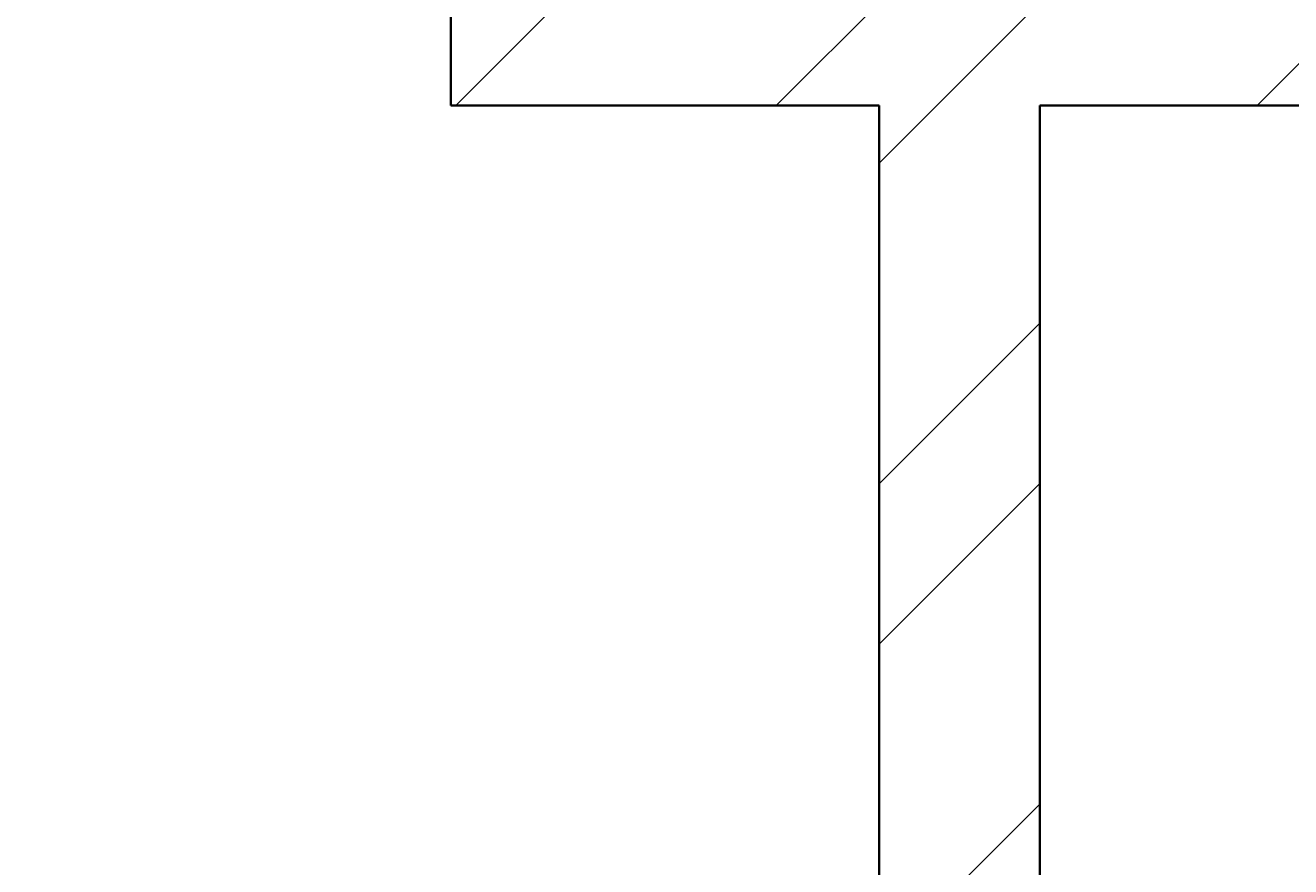
# Model space of a CAD drawing. Units: inches. Extents: x 1885 to 2748, y 783 to 2421.
# Tile 76 of 117: x 1969 to 2004, y 2144 to 2167. Entities that reach past the tile are written whole.
import ezdxf

# ---------------------------------------------------------------- set-up
doc = ezdxf.new("R2010")
doc.units = ezdxf.units.IN
doc.layers.add('A-ANNO-DIMS', color=2, linetype='Continuous', lineweight=18)
doc.layers.add('A-WALL', color=7, linetype='Continuous', lineweight=35)
doc.layers.add('A-WALL-PATT', color=85, linetype='Continuous', lineweight=13, true_color=0x58ba48)
doc.styles.get("Standard").update_dxf_attribs({"font": 'arial.ttf'})
doc.dimstyles.get("Standard").update_dxf_attribs({"dimtxt": 0.18, "dimasz": 0.18, "dimexe": 0.18, "dimexo": 0.0625, "dimgap": 0.09, "dimtad": 0, "dimtih": 1, "dimtoh": 1, "dimdec": 4, "dimzin": 0, "dimdsep": 46, "dimtxsty": 'Standard', "dimcen": 0.09, "dimadec": 0, "dimazin": 0, "dimtfac": 1, "dimtdec": 4, "dimtofl": 0, "dimtmove": 0, "dimatfit": 3, "dimfxl": 1, "dimtolj": 1, "dimtzin": 0, "dimarcsym": 0})

# ---------------------------------------------------------------- blocks, each defined once
blk = doc.blocks.new('*D48')
at = {"layer": 'A-ANNO-DIMS', "color": 0, "lineweight": -2, "transparency": 16777216}
for p, q in [((1980.711, 2348.006), (1902.844, 2348.006)), ((1903.024, 2347.826), (1903.024, 2114.937)), ((1903.024, 1881.686), (1903.024, 2114.574)), ((2016.711, 1881.506), (1902.844, 1881.506))]:
    blk.add_line(p, q, dxfattribs=at)
at = {"layer": 'A-ANNO-DIMS', "color": 0, "transparency": 16777216}
for points in [[(1902.994, 2347.826), (1903.054, 2347.826), (1903.024, 2348.006)], [(1902.994, 1881.686), (1903.054, 1881.686), (1903.024, 1881.506)]]:
    blk.add_solid(points, dxfattribs=at)
at = {"layer": 'Defpoints', "color": 0, "transparency": 16777216}
for p in [(1903.024, 2348.006), (1980.774, 2348.006), (2016.774, 1881.506)]:
    blk.add_point(p, dxfattribs=at)
at = {"layer": 'A-ANNO-DIMS', "color": 0, "transparency": 16777216, "insert": (1903.024, 2114.756), "char_height": 0.18, "attachment_point": 5}
blk.add_mtext('\\A1;466.5', dxfattribs=at)

msp = doc.modelspace()

# ---------------------------------------------------------------- hatches: boundary and pattern name
at = {"layer": 'A-WALL-PATT'}
h = msp.add_hatch(dxfattribs=at)
h.set_pattern_fill('ANSI32', color=256)
h.paths.add_polyline_path([(2007.772, 2318.006), (1980.774, 2318.006), (1980.774, 2281.215), (1985.274, 2281.215), (1985.274, 2313.506), (2007.772, 2313.506), (2007.772, 2315.756)])
h.paths.add_polyline_path([(2094.324, 2318.006), (2067.772, 2318.006), (2067.772, 2313.506), (2094.324, 2313.506), (2094.324, 2315.756)])
h.paths.add_polyline_path([(2131.367, 2315.756), (2131.367, 2318.006), (2131.189, 2318.006), (2112.609, 2318.006), (2112.609, 2313.506), (2117.274, 2313.506), (2117.274, 2255.201), (2121.774, 2255.201), (2121.774, 2313.506), (2131.367, 2313.506)])
h.paths.add_polyline_path([(2190.512, 2318.006), (2155.367, 2318.006), (2155.367, 2313.506), (2169.774, 2313.506), (2169.774, 2229.506), (2121.774, 2229.506), (2121.774, 2233.451), (2119.524, 2233.451), (2117.274, 2233.451), (2117.274, 2201.101), (2121.774, 2201.101), (2121.774, 2225.006), (2169.774, 2225.006), (2169.774, 2165.006), (2306.274, 2165.006), (2306.274, 2066.006), (2310.774, 2066.006), (2344.274, 2066.006), (2486.274, 2066.006), (2486.274, 1886.006), (2483.02, 1886.006), (2483.02, 1881.506), (2486.274, 1881.506), (2486.274, 1880.678), (2490.774, 1880.678), (2490.774, 2070.506), (2344.274, 2070.506), (2310.774, 2070.506), (2310.774, 2165.006), (2310.774, 2173.636), (2308.524, 2173.636), (2306.274, 2173.636), (2306.274, 2169.506), (2174.274, 2169.506), (2174.274, 2313.506), (2190.512, 2313.506), (2190.512, 2315.756)])
h.paths.add_polyline_path([(1985.274, 2221.215), (1980.774, 2221.215), (1980.774, 2165.006), (1992.774, 2165.006), (1992.774, 2141.927), (1997.274, 2141.927), (1997.274, 2165.006), (2117.274, 2165.006), (2117.274, 2163.126), (2121.774, 2163.126), (2121.774, 2172.734), (2119.524, 2172.734), (2117.274, 2172.734), (2117.274, 2169.506), (1985.274, 2169.506)])
h.paths.add_polyline_path([(1997.274, 2105.927), (1992.774, 2105.927), (1992.774, 2070.506), (2016.774, 2070.506), (2016.774, 2059.123), (2019.024, 2059.123), (2021.274, 2059.123), (2021.274, 2070.506), (2117.274, 2070.506), (2117.274, 2022.506), (2114.423, 2022.506), (2114.423, 2018.006), (2123.627, 2018.006), (2123.627, 2020.256), (2123.627, 2022.506), (2121.774, 2022.506), (2121.774, 2142.587), (2119.524, 2142.587), (2117.274, 2142.587), (2117.274, 2075.006), (1997.274, 2075.006)])
h.paths.add_polyline_path([(2092.029, 2020.256), (2092.029, 2022.506), (2021.274, 2022.506), (2021.274, 2035.123), (2016.774, 2035.123), (2016.774, 2018.006), (2016.774, 1978.784), (2021.274, 1978.784), (2021.274, 2018.006), (2092.029, 2018.006)])
h.paths.add_polyline_path([(2260.938, 2022.506), (2153.105, 2022.506), (2153.105, 2020.256), (2153.105, 2018.006), (2155.274, 2018.006), (2155.274, 1886.006), (2107.629, 1886.006), (2107.629, 1881.506), (2182.911, 1881.506), (2182.911, 1883.756), (2182.911, 1886.006), (2159.774, 1886.006), (2159.774, 2018.006), (2260.938, 2018.006), (2260.938, 2020.256)])
h.paths.add_polyline_path([(2047.629, 1883.756), (2047.629, 1886.006), (2021.274, 1886.006), (2021.274, 1918.784), (2019.024, 1918.784), (2016.774, 1918.784), (2016.774, 1881.506), (2047.629, 1881.506)])
h.paths.add_polyline_path([(2306.361, 1883.756), (2306.361, 1886.006), (2296.274, 1886.006), (2296.274, 1982.006), (2316.535, 1982.006), (2316.535, 1984.256), (2316.535, 1986.506), (2296.274, 1986.506), (2296.274, 2022.506), (2289.276, 2022.506), (2289.276, 2018.006), (2291.774, 2018.006), (2291.774, 1886.006), (2242.911, 1886.006), (2242.911, 1881.506), (2306.361, 1881.506)], flags=17)
h.paths.add_polyline_path([(1985.274, 1843.006), (2021.6, 1843.006), (2021.534, 1845.441), (2021.477, 1847.506), (1980.774, 1847.506), (1980.774, 1809.446), (1985.274, 1809.446)])
h.paths.add_polyline_path([(2131.482, 1845.256), (2131.482, 1847.506), (2081.534, 1847.506), (2081.534, 1843.006), (2117.274, 1843.006), (2117.274, 1784.147), (2119.524, 1784.147), (2121.774, 1784.147), (2121.774, 1843.006), (2131.482, 1843.006)])
h.paths.add_polyline_path([(2203.886, 1847.506), (2155.482, 1847.506), (2155.482, 1843.006), (2169.774, 1843.006), (2169.774, 1759.006), (2121.774, 1759.006), (2121.774, 1761.457), (2117.274, 1761.457), (2117.274, 1730.429), (2121.774, 1730.429), (2121.774, 1754.506), (2177.421, 1754.506), (2177.421, 1756.756), (2177.421, 1759.006), (2174.274, 1759.006), (2174.274, 1843.006), (2203.886, 1843.006)])
h.paths.add_polyline_path([(2335.554, 1845.256), (2335.554, 1847.506), (2239.886, 1847.506), (2239.886, 1843.006), (2306.274, 1843.006), (2306.274, 1759.006), (2199.486, 1759.006), (2199.486, 1754.506), (2310.774, 1754.506), (2310.774, 1843.006), (2335.554, 1843.006)])
h.paths.add_polyline_path([(2348.774, 2022.506), (2344.274, 2022.506), (2344.274, 1986.506), (2341.681, 1986.506), (2341.681, 1982.006), (2344.274, 1982.006), (2344.274, 1886.006), (2330.361, 1886.006), (2330.361, 1881.506), (2361.627, 1881.506), (2361.627, 1883.756), (2361.627, 1886.006), (2348.774, 1886.006)], flags=17)
h.paths.add_polyline_path([(2283.251, 2315.756), (2283.251, 2318.006), (2238.512, 2318.006), (2238.512, 2313.506), (2283.251, 2313.506)], flags=17)
h.paths.add_polyline_path([(2363.274, 2348.006), (2388.677, 2348.006), (2388.677, 2350.256), (2388.677, 2352.506), (2358.774, 2352.506), (2358.774, 2348.006), (2358.774, 2318.006), (2344.481, 2318.006), (2344.481, 2313.506), (2358.774, 2313.506), (2358.774, 2229.506), (2310.774, 2229.506), (2310.774, 2231.952), (2306.274, 2231.952), (2306.274, 2205.611), (2310.774, 2205.611), (2310.774, 2225.006), (2358.774, 2225.006), (2358.774, 2211.506), (2452.329, 2211.506), (2452.329, 2213.756), (2452.329, 2216.006), (2363.274, 2216.006), (2363.274, 2318.006)])
h.paths.add_polyline_path([(2310.774, 2313.506), (2320.481, 2313.506), (2320.481, 2315.756), (2320.481, 2318.006), (2302.728, 2318.006), (2302.728, 2313.506), (2306.274, 2313.506), (2306.274, 2251.076), (2310.774, 2251.076)], flags=17)
h.paths.add_polyline_path([(2490.774, 2352.506), (2486.274, 2352.506), (2448.677, 2352.506), (2448.677, 2348.006), (2486.274, 2348.006), (2486.274, 2318.006), (2486.274, 2216.006), (2481.78, 2216.006), (2481.78, 2211.506), (2486.274, 2211.506), (2486.274, 2165.006), (2493.289, 2165.006), (2493.289, 2167.256), (2493.289, 2169.506), (2490.774, 2169.506), (2490.774, 2313.506), (2494.429, 2313.506), (2494.429, 2318.006), (2490.774, 2318.006)])
h.paths.add_polyline_path([(2534.653, 2318.006), (2515.691, 2318.006), (2515.691, 2313.506), (2534.653, 2313.506), (2534.653, 2315.756)])
h.paths.add_polyline_path([(2618.274, 2318.006), (2594.653, 2318.006), (2594.653, 2313.506), (2613.774, 2313.506), (2613.774, 2281.706), (2618.274, 2281.706)])
h.paths.add_polyline_path([(2618.274, 2221.706), (2613.774, 2221.706), (2613.774, 2169.506), (2554.019, 2169.506), (2554.019, 2165.006), (2613.774, 2165.006), (2613.774, 2152.878), (2618.274, 2152.878)])
h.paths.add_polyline_path([(2618.274, 2128.878), (2616.024, 2128.878), (2613.774, 2128.878), (2613.774, 2117.006), (2529.774, 2117.006), (2529.774, 2165.006), (2532.848, 2165.006), (2532.848, 2169.506), (2522.867, 2169.506), (2522.867, 2165.006), (2525.274, 2165.006), (2525.274, 2117.006), (2525.274, 2112.506), (2525.274, 2108.576), (2529.774, 2108.576), (2529.774, 2112.506), (2613.774, 2112.506), (2613.774, 2080.19), (2618.274, 2080.19)])
h.paths.add_polyline_path([(2618.274, 2044.19), (2616.024, 2044.19), (2613.774, 2044.19), (2613.774, 2015.506), (2529.774, 2015.506), (2529.774, 2088.582), (2527.524, 2088.582), (2525.274, 2088.582), (2525.274, 2011.006), (2613.774, 2011.006), (2613.774, 1956.755), (2618.274, 1956.755)])
h.paths.add_polyline_path([(2618.274, 1881.506), (2618.274, 1896.755), (2613.774, 1896.755), (2613.774, 1881.506), (2613.774, 1847.506), (2592.715, 1847.506), (2592.715, 1843.006), (2613.774, 1843.006), (2613.774, 1765.006), (2613.774, 1760.506), (2609.621, 1760.506), (2609.621, 1756.006), (2613.774, 1756.006), (2613.774, 1660.006), (2608.544, 1660.006), (2608.544, 1655.506), (2613.774, 1655.506), (2613.774, 1508.158), (2618.274, 1508.158)])
h.paths.add_polyline_path([(2565.774, 1843.006), (2568.997, 1843.006), (2568.997, 1847.506), (2490.774, 1847.506), (2490.774, 1849.7), (2488.524, 1849.7), (2486.274, 1849.7), (2486.274, 1847.506), (2477.274, 1847.506), (2477.274, 1838.506), (2477.274, 1821.493), (2486.274, 1821.493), (2486.274, 1838.506), (2561.274, 1838.506), (2561.274, 1765.006), (2486.274, 1765.006), (2486.274, 1786.157), (2477.274, 1786.157), (2477.274, 1765.006), (2477.274, 1756.006), (2486.274, 1756.006), (2565.774, 1756.006), (2585.621, 1756.006), (2585.621, 1758.256), (2585.621, 1760.506), (2565.774, 1760.506), (2565.774, 1765.006)])
h.paths.add_polyline_path([(2486.274, 1651.006), (2561.274, 1651.006), (2561.274, 1567.006), (2486.274, 1567.006), (2486.274, 1591.321), (2477.274, 1591.321), (2477.274, 1567.006), (2477.274, 1558.006), (2477.274, 1555.439), (2481.774, 1555.439), (2481.774, 1558.006), (2568.653, 1558.006), (2568.653, 1560.256), (2568.653, 1562.506), (2565.774, 1562.506), (2565.774, 1655.506), (2584.544, 1655.506), (2584.544, 1657.756), (2584.544, 1660.006), (2565.774, 1660.006), (2486.274, 1660.006), (2477.274, 1660.006), (2477.274, 1651.006), (2477.274, 1632.989), (2486.274, 1632.989)])
h.paths.add_polyline_path([(2449.967, 1883.756), (2449.967, 1886.006), (2421.627, 1886.006), (2421.627, 1881.506), (2449.967, 1881.506)], flags=17)
h.paths.add_polyline_path([(2447.274, 1847.506), (2395.554, 1847.506), (2395.554, 1843.006), (2442.774, 1843.006), (2442.774, 1809.27), (2447.274, 1809.27)])
h.paths.add_polyline_path([(1985.274, 1749.446), (1980.774, 1749.446), (1980.774, 1694.504), (1985.274, 1694.504), (1985.274, 1694.506), (1986.897, 1694.506), (1986.897, 1697.78), (1986.897, 1699.006), (1985.274, 1699.006)])
h.paths.add_polyline_path([(2152.774, 1699.006), (2121.774, 1699.006), (2121.774, 1703.668), (2119.524, 1703.668), (2117.274, 1703.668), (2117.274, 1699.006), (2009.219, 1699.006), (2009.219, 1694.506), (2148.274, 1694.506), (2148.274, 1692.631), (2152.774, 1692.631)])
h.paths.add_polyline_path([(2016.274, 1694.506), (2011.774, 1694.506), (2011.774, 1558.006), (2040.806, 1558.006), (2040.806, 1560.256), (2040.806, 1562.506), (2016.274, 1562.506)])
h.paths.add_polyline_path([(2152.774, 1663.017), (2150.524, 1663.017), (2148.274, 1663.017), (2148.274, 1562.506), (2100.806, 1562.506), (2100.806, 1558.006), (2165.119, 1558.006), (2165.119, 1560.256), (2165.119, 1562.506), (2152.774, 1562.506), (2152.774, 1610.506), (2224.774, 1610.506), (2224.774, 1607.99), (2229.274, 1607.99), (2229.274, 1615.006), (2152.774, 1615.006)])
h.paths.add_polyline_path([(2238.613, 1560.256), (2238.613, 1562.506), (2229.274, 1562.506), (2229.274, 1588.756), (2227.024, 1588.763), (2224.774, 1588.771), (2224.774, 1562.506), (2189.119, 1562.506), (2189.119, 1558.006), (2238.613, 1558.006)])
h.paths.add_polyline_path([(2336.024, 1560.256), (2336.024, 1562.506), (2310.774, 1562.506), (2310.774, 1656.347), (2308.524, 1656.347), (2306.274, 1656.347), (2306.274, 1562.506), (2286.613, 1562.506), (2286.613, 1558.006), (2336.024, 1558.006)])
h.paths.add_polyline_path([(2447.274, 1690.968), (2445.024, 1690.968), (2442.774, 1690.968), (2442.774, 1687.006), (2306.274, 1687.006), (2306.274, 1680.75), (2310.774, 1680.75), (2310.774, 1682.506), (2442.774, 1682.506), (2442.774, 1562.506), (2396.024, 1562.506), (2396.024, 1558.006), (2447.274, 1558.006)])
h.paths.add_polyline_path([(2447.274, 1749.27), (2445.024, 1749.27), (2442.774, 1749.27), (2442.774, 1717.232), (2447.274, 1717.232)])
h.paths.add_polyline_path([(2044.674, 1521.756), (2044.674, 1524.006), (2007.274, 1524.006), (2007.274, 1503.49), (2009.524, 1503.49), (2011.774, 1503.49), (2011.774, 1519.506), (2044.674, 1519.506)])
h.paths.add_polyline_path([(2177.969, 1521.756), (2177.969, 1524.006), (2104.674, 1524.006), (2104.674, 1519.506), (2145.774, 1519.506), (2145.774, 1387.506), (2143.37, 1387.506), (2143.37, 1383.006), (2251.585, 1383.006), (2251.585, 1385.256), (2251.585, 1387.506), (2150.274, 1387.506), (2150.274, 1519.506), (2177.969, 1519.506)])
h.paths.add_polyline_path([(2298.704, 1524.006), (2237.969, 1524.006), (2237.969, 1519.506), (2282.274, 1519.506), (2282.274, 1387.506), (2279.683, 1387.506), (2279.683, 1383.006), (2286.774, 1383.006), (2286.774, 1419.006), (2312.451, 1419.006), (2312.451, 1421.256), (2312.451, 1423.506), (2286.774, 1423.506), (2286.774, 1519.506), (2298.704, 1519.506), (2298.704, 1521.722)], flags=17)
h.paths.add_polyline_path([(2361.897, 1521.756), (2361.897, 1524.006), (2322.704, 1524.006), (2322.704, 1519.506), (2334.774, 1519.506), (2334.774, 1423.506), (2331.93, 1423.506), (2331.93, 1419.006), (2334.774, 1419.006), (2334.774, 1387.506), (2334.774, 1383.228), (2339.274, 1383.228), (2339.274, 1387.506), (2339.274, 1519.506), (2361.897, 1519.506)], flags=17)
h.paths.add_polyline_path([(2447.274, 1521.756), (2447.274, 1524.006), (2421.897, 1524.006), (2421.897, 1519.506), (2447.274, 1519.506)], flags=17)
h.paths.add_polyline_path([(2481.774, 1529.6), (2479.524, 1529.6), (2477.274, 1529.6), (2477.274, 1524.006), (2474.489, 1524.006), (2474.489, 1519.506), (2477.274, 1519.506), (2477.274, 1334.506), (2296.774, 1334.506), (2296.774, 1240.506), (2160.274, 1240.506), (2160.274, 1180.506), (2112.274, 1180.506), (2112.274, 1207.692), (2110.024, 1207.692), (2107.774, 1207.692), (2107.774, 1171.609), (2112.274, 1171.609), (2112.274, 1176.006), (2160.274, 1176.006), (2160.274, 1092.006), (2144.221, 1092.006), (2144.221, 1087.506), (2189.497, 1087.506), (2189.497, 1089.756), (2189.497, 1092.006), (2164.774, 1092.006), (2164.774, 1236.006), (2296.774, 1236.006), (2296.774, 1231.912), (2301.274, 1231.912), (2301.274, 1330.006), (2481.774, 1330.006), (2481.774, 1387.506)])
h.paths.add_polyline_path([(2618.274, 1448.158), (2613.774, 1448.158), (2613.774, 1382.506), (2529.774, 1382.506), (2525.274, 1382.506), (2525.274, 1307.062), (2529.774, 1307.062), (2529.774, 1378.006), (2613.774, 1378.006), (2613.774, 1354.988), (2618.274, 1354.988)])
h.paths.add_polyline_path([(2618.274, 1318.988), (2613.774, 1318.988), (2613.774, 1281.006), (2529.774, 1281.006), (2529.774, 1283.786), (2527.524, 1283.786), (2525.274, 1283.786), (2525.274, 1228.506), (2516.794, 1228.506), (2516.794, 1224.006), (2533.484, 1224.006), (2533.484, 1226.256), (2533.484, 1228.506), (2529.774, 1228.506), (2529.774, 1276.506), (2613.774, 1276.506), (2613.774, 1266.02), (2618.274, 1266.02)])
h.paths.add_polyline_path([(2618.274, 1134.964), (2613.774, 1134.964), (2613.774, 1092.006), (2594.545, 1092.006), (2594.545, 1087.506), (2618.274, 1087.506)])
h.paths.add_polyline_path([(2534.545, 1092.006), (2509.765, 1092.006), (2509.765, 1087.506), (2534.545, 1087.506), (2534.545, 1089.756)])
h.paths.add_polyline_path([(2481.274, 1224.006), (2484.117, 1224.006), (2484.117, 1226.256), (2484.117, 1228.506), (2476.774, 1228.506), (2476.774, 1198.506), (2471.61, 1198.506), (2471.61, 1194.006), (2476.774, 1194.006), (2476.774, 1062.006), (2436.894, 1062.006), (2436.894, 1057.506), (2476.774, 1057.506), (2481.274, 1057.506), (2481.274, 1062.006), (2481.274, 1087.506), (2485.354, 1087.506), (2485.354, 1089.756), (2485.354, 1092.006), (2481.274, 1092.006), (2481.274, 1117.506)])
h.paths.add_polyline_path([(2439.898, 1198.506), (2349.274, 1198.506), (2349.274, 1194.006), (2349.274, 1180.506), (2301.274, 1180.506), (2301.274, 1201.896), (2299.024, 1201.896), (2296.774, 1201.896), (2296.774, 1172.335), (2299.024, 1172.335), (2301.274, 1172.335), (2301.274, 1176.006), (2349.274, 1176.006), (2349.274, 1092.006), (2334.452, 1092.006), (2334.452, 1087.506), (2349.274, 1087.506), (2349.274, 1057.506), (2353.774, 1057.506), (2376.894, 1057.506), (2376.894, 1059.756), (2376.894, 1062.006), (2353.774, 1062.006), (2353.774, 1087.506), (2353.774, 1180.506), (2353.774, 1194.006), (2439.898, 1194.006), (2439.898, 1196.256)])
h.paths.add_polyline_path([(2270.596, 1089.756), (2270.596, 1092.006), (2249.497, 1092.006), (2249.497, 1087.506), (2270.596, 1087.506)], flags=17)
h.paths.add_polyline_path([(2310.452, 1092.006), (2301.274, 1092.006), (2301.274, 1153.292), (2296.774, 1153.292), (2296.774, 1092.006), (2293.786, 1092.006), (2293.786, 1087.506), (2310.452, 1087.506), (2310.452, 1089.756)], flags=17)
h.paths.add_polyline_path([(2112.274, 1150.328), (2110.024, 1150.328), (2107.774, 1150.328), (2107.774, 1092.006), (2104.465, 1092.006), (2104.465, 1087.506), (2120.221, 1087.506), (2120.221, 1089.756), (2120.221, 1092.006), (2112.274, 1092.006)])
h.paths.add_polyline_path([(2082.172, 1092.006), (2058.144, 1092.006), (2058.144, 1087.506), (2082.172, 1087.506), (2082.172, 1089.756)])
h.paths.add_polyline_path([(1975.774, 1145.638), (1971.274, 1145.638), (1971.274, 1087.506), (1980.774, 1087.506), (1998.144, 1087.506), (1998.144, 1089.756), (1998.144, 1092.006), (1985.274, 1092.006), (1975.774, 1092.006)])
h.paths.add_polyline_path([(2112.274, 1244.385), (2110.024, 1244.385), (2107.774, 1244.385), (2107.774, 1240.506), (1992.274, 1240.506), (1992.274, 1271.008), (1987.774, 1271.008), (1987.774, 1240.506), (1980.774, 1240.506), (1975.774, 1240.506), (1971.274, 1240.506), (1971.274, 1205.638), (1975.774, 1205.638), (1975.774, 1236.006), (2107.774, 1236.006), (2107.774, 1233.444), (2112.274, 1233.444), (2112.274, 1236.006)])
h.paths.add_polyline_path([(2112.274, 1383.006), (2114.783, 1383.006), (2114.783, 1385.256), (2114.783, 1387.506), (2102.476, 1387.506), (2102.476, 1383.006), (2107.774, 1383.006), (2107.774, 1335.006), (2011.774, 1335.006), (2011.774, 1349.939), (2007.274, 1349.939), (2007.274, 1335.006), (1987.774, 1335.006), (1987.774, 1330.506), (1987.774, 1307.008), (1992.274, 1307.008), (1992.274, 1330.506), (2007.274, 1330.506), (2107.774, 1330.506), (2107.774, 1264.711), (2112.274, 1264.711)])
h.paths.add_polyline_path([(2077.857, 1387.506), (2011.774, 1387.506), (2011.774, 1390.036), (2009.524, 1390.036), (2007.274, 1390.036), (2007.274, 1373.939), (2011.774, 1373.939), (2011.774, 1383.006), (2077.857, 1383.006)])
h.paths.add_polyline_path([(2011.774, 1443.49), (2007.274, 1443.49), (2007.274, 1410.248), (2011.774, 1410.248)])

# ---------------------------------------------------------------- linework, layer by layer
at = {"layer": 'A-WALL'}
for p, q in [((1980.774, 2221.215), (1980.774, 2165.006)), ((1980.774, 2165.006), (1992.774, 2165.006)), ((1992.774, 2165.006), (1992.774, 2141.927)), ((1997.274, 2165.006), (1997.274, 2141.927)), ((1997.274, 2165.006), (2117.274, 2165.006))]:
    msp.add_line(p, q, dxfattribs=at)

# ---------------------------------------------------------------- dimensions: what is measured, and where the dimension line sits
at = {"layer": 'A-ANNO-DIMS'}
dim = msp.add_linear_dim(base=(1903.024, 2348.006), p1=(2016.774, 1881.506), p2=(1980.774, 2348.006), angle=90, dimstyle='Standard', override={"dimdec": 1, "dimlfac": 1, "dimrnd": 0, "dimzin": 0, "dimdsep": 46, "dimlunit": 2}, dxfattribs=at)
dim.commit()
dim.dimension.update_dxf_attribs({"geometry": '*D48', "text_midpoint": (1903.024, 2114.756)})

doc.saveas('drawing.dxf')
